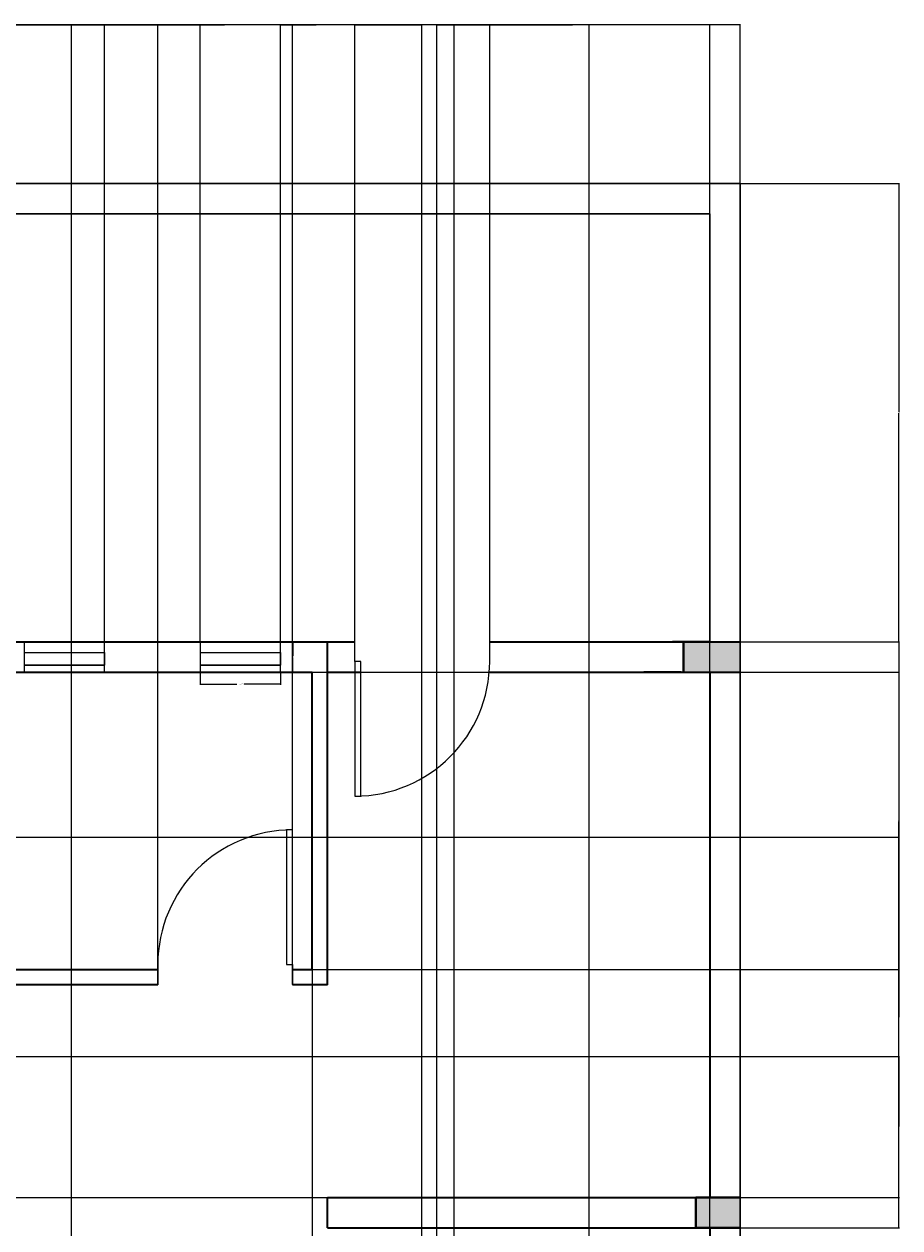
# Model space of a CAD drawing. Units: inches. Extents: x 1210 to 1836, y 84 to 1122.
# Tile 5 of 5: x 1576 to 1836, y 764 to 1122. Entities that reach past the tile are written whole.
import ezdxf

# ---------------------------------------------------------------- set-up
doc = ezdxf.new("R2010")
doc.units = ezdxf.units.IN
doc.header["$MEASUREMENT"] = 0
for name, color, linetype, lineweight in [('A-ANNO-DIMS', 2, 'Continuous', 18), ('A-COLS', 7, 'Continuous', 40), ('A-COLS-PATT', 6, 'Continuous', 13), ('A-GLAZ', 4, 'Continuous', 18), ('A-WALL', 7, 'Continuous', 35), ('C-PROP', 32, 'Continuous', 30), ('DOORS', 24, 'Continuous', 25)]:
    doc.layers.add(name, color=color, linetype=linetype, lineweight=lineweight)
doc.styles.get("Standard").update_dxf_attribs({"font": 'arial.ttf'})
doc.dimstyles.get("Standard").update_dxf_attribs({"dimtxt": 0.18, "dimasz": 0.18, "dimexe": 0.18, "dimexo": 0.0625, "dimgap": 0.09, "dimtad": 0, "dimtih": 1, "dimtoh": 1, "dimdec": 4, "dimzin": 0, "dimdsep": 46, "dimtxsty": 'Standard', "dimcen": 0.09, "dimadec": 0, "dimazin": 0, "dimtfac": 1, "dimtdec": 4, "dimtofl": 0, "dimtmove": 0, "dimatfit": 3, "dimfxl": 1, "dimtolj": 1, "dimtzin": 0, "dimarcsym": 0})

# ---------------------------------------------------------------- blocks, each defined once
blk = doc.blocks.new('*U3')
for p, q in [((0, 0), (0, -6)), ((-40, 0), (-40, -6))]:
    blk.add_line(p, q)
blk.add_lwpolyline([(0, 0), (0, 40), (-1.75, 40), (-1.75, 0)], close=True)
blk.add_arc((0, 0), 40, 90, 180)
blk = doc.blocks.new('*U4')
for p, q in [((0, 0), (0, 6)), ((40, 0), (40, 6))]:
    blk.add_line(p, q)
blk.add_lwpolyline([(0, 0), (0, -40), (1.75, -40), (1.75, 0)], close=True)
blk.add_arc((0, 0), 40, 270, 0)
blk = doc.blocks.new('WIN-24IN')
for p, q in [((0, 9), (0, 0)), ((23.85, 0), (23.85, 9)), ((0.11, 5.82), (23.85, 5.82)), ((23.85, 5.82), (23.85, 2.02)), ((23.85, 2.02), (0, 2.02)), ((0, 2.02), (23.85, 2.02)), ((0, 0), (23.85, 0))]:
    blk.add_line(p, q)
blk = doc.blocks.new('*D20')
at = {"layer": 'A-ANNO-DIMS', "color": 0, "lineweight": -2, "transparency": 16777216}
for p, q in [((1628.07, 929.15), (1628.07, 925.46)), ((1651.92, 929.15), (1651.92, 925.46)), ((1628.25, 925.64), (1638.88, 925.64)), ((1651.74, 925.64), (1641.12, 925.64))]:
    blk.add_line(p, q, dxfattribs=at)
at = {"layer": 'A-ANNO-DIMS', "color": 0, "transparency": 16777216}
for points in [[(1628.25, 925.67), (1628.25, 925.61), (1628.07, 925.64)], [(1651.74, 925.67), (1651.74, 925.61), (1651.92, 925.64)]]:
    blk.add_solid(points, dxfattribs=at)
at = {"layer": 'Defpoints', "color": 0, "transparency": 16777216}
for p in [(1628.07, 929.21), (1651.92, 929.21), (1651.92, 925.64)]:
    blk.add_point(p, dxfattribs=at)
at = {"layer": 'A-ANNO-DIMS', "color": 0, "transparency": 16777216, "insert": (1640, 925.64), "char_height": 0.18, "attachment_point": 5}
blk.add_mtext('\\A1;WINDOW 24 TYP.', dxfattribs=at)
blk = doc.blocks.new('*D21')
at = {"layer": 'A-ANNO-DIMS', "color": 0, "lineweight": -2, "transparency": 16777216}
for p, q in [((1651.99, 938.21), (1655.68, 938.21)), ((1655.5, 938.03), (1655.5, 933.9)), ((1655.5, 929.39), (1655.5, 933.53)), ((1651.99, 929.21), (1655.68, 929.21))]:
    blk.add_line(p, q, dxfattribs=at)
at = {"layer": 'A-ANNO-DIMS', "color": 0, "transparency": 16777216}
for points in [[(1655.47, 938.03), (1655.53, 938.03), (1655.5, 938.21)], [(1655.47, 929.39), (1655.53, 929.39), (1655.5, 929.21)]]:
    blk.add_solid(points, dxfattribs=at)
at = {"layer": 'Defpoints', "color": 0, "transparency": 16777216}
for p in [(1651.92, 938.21), (1655.5, 938.21), (1651.92, 929.21)]:
    blk.add_point(p, dxfattribs=at)
at = {"layer": 'A-ANNO-DIMS', "color": 0, "transparency": 16777216, "insert": (1655.5, 933.71), "char_height": 0.18, "attachment_point": 5}
blk.add_mtext('\\A1;9 TYP.', dxfattribs=at)
blk = doc.blocks.new('*D22')
at = {"layer": 'A-ANNO-DIMS', "color": 0, "lineweight": -2, "transparency": 16777216}
for p, q in [((1257.32, 1074.28), (1257.32, 1121.57)), ((1257.5, 1121.39), (1522.55, 1121.39)), ((1788.14, 1121.39), (1523.1, 1121.39)), ((1788.32, 1074.28), (1788.32, 1121.57))]:
    blk.add_line(p, q, dxfattribs=at)
at = {"layer": 'A-ANNO-DIMS', "color": 0, "transparency": 16777216}
for points in [[(1257.5, 1121.42), (1257.5, 1121.36), (1257.32, 1121.39)], [(1788.14, 1121.42), (1788.14, 1121.36), (1788.32, 1121.39)]]:
    blk.add_solid(points, dxfattribs=at)
at = {"layer": 'Defpoints', "color": 0, "transparency": 16777216}
for p in [(1788.32, 1121.39), (1257.32, 1074.21), (1788.32, 1074.21)]:
    blk.add_point(p, dxfattribs=at)
at = {"layer": 'A-ANNO-DIMS', "color": 0, "transparency": 16777216, "insert": (1522.82, 1121.39), "char_height": 0.18, "attachment_point": 5}
blk.add_mtext('\\A1;531', dxfattribs=at)
blk = doc.blocks.new('*D24')
at = {"layer": 'A-ANNO-DIMS', "color": 0, "lineweight": -2, "transparency": 16777216}
for p, q in [((1788.39, 1074.21), (1835.68, 1074.21)), ((1835.5, 1074.03), (1835.5, 1006.4)), ((1835.5, 938.39), (1835.5, 1006.03)), ((1788.39, 938.21), (1835.68, 938.21))]:
    blk.add_line(p, q, dxfattribs=at)
at = {"layer": 'A-ANNO-DIMS', "color": 0, "transparency": 16777216}
for points in [[(1835.47, 1074.03), (1835.53, 1074.03), (1835.5, 1074.21)], [(1835.47, 938.39), (1835.53, 938.39), (1835.5, 938.21)]]:
    blk.add_solid(points, dxfattribs=at)
at = {"layer": 'Defpoints', "color": 0, "transparency": 16777216}
for p in [(1788.32, 1074.21), (1788.32, 938.21), (1835.5, 938.21)]:
    blk.add_point(p, dxfattribs=at)
at = {"layer": 'A-ANNO-DIMS', "color": 0, "transparency": 16777216, "insert": (1835.5, 1006.21), "char_height": 0.18, "attachment_point": 5}
blk.add_mtext('\\A1;136', dxfattribs=at)
blk = doc.blocks.new('*D25')
at = {"layer": 'A-ANNO-DIMS', "color": 0, "lineweight": -2, "transparency": 16777216}
for p, q in [((1788.39, 938.21), (1835.68, 938.21)), ((1835.5, 938.03), (1835.5, 851.39)), ((1835.5, 764.39), (1835.5, 851.03)), ((1788.39, 764.21), (1835.68, 764.21))]:
    blk.add_line(p, q, dxfattribs=at)
at = {"layer": 'A-ANNO-DIMS', "color": 0, "transparency": 16777216}
for points in [[(1835.47, 938.03), (1835.53, 938.03), (1835.5, 938.21)], [(1835.47, 764.39), (1835.53, 764.39), (1835.5, 764.21)]]:
    blk.add_solid(points, dxfattribs=at)
at = {"layer": 'Defpoints', "color": 0, "transparency": 16777216}
for p in [(1788.32, 938.21), (1788.32, 764.21), (1835.5, 764.21)]:
    blk.add_point(p, dxfattribs=at)
at = {"layer": 'A-ANNO-DIMS', "color": 0, "transparency": 16777216, "insert": (1835.5, 851.21), "char_height": 0.18, "attachment_point": 5}
blk.add_mtext('\\A1;174', dxfattribs=at)
blk = doc.blocks.new('*D36')
at = {"layer": 'A-ANNO-DIMS', "color": 0, "lineweight": -2, "transparency": 16777216}
for p, q in [((1552.32, 840.82), (1552.32, 83.86)), ((1661.32, 840.82), (1661.32, 83.86)), ((1552.5, 84.04), (1606.54, 84.04)), ((1661.14, 84.04), (1607.1, 84.04))]:
    blk.add_line(p, q, dxfattribs=at)
at = {"layer": 'A-ANNO-DIMS', "color": 0, "transparency": 16777216}
for points in [[(1552.5, 84.07), (1552.5, 84.01), (1552.32, 84.04)], [(1661.14, 84.07), (1661.14, 84.01), (1661.32, 84.04)]]:
    blk.add_solid(points, dxfattribs=at)
at = {"layer": 'Defpoints', "color": 0, "transparency": 16777216}
for p in [(1552.32, 840.89), (1661.32, 840.89), (1661.32, 84.04)]:
    blk.add_point(p, dxfattribs=at)
at = {"layer": 'A-ANNO-DIMS', "color": 0, "transparency": 16777216, "insert": (1606.82, 84.04), "char_height": 0.18, "attachment_point": 5}
blk.add_mtext('\\A1;109', dxfattribs=at)
blk = doc.blocks.new('*D37')
at = {"layer": 'A-ANNO-DIMS', "color": 0, "lineweight": -2, "transparency": 16777216}
for p, q in [((1661.39, 929.21), (1835.68, 929.21)), ((1835.5, 929.03), (1835.5, 885.23)), ((1835.5, 841.07), (1835.5, 884.87)), ((1661.39, 840.89), (1835.68, 840.89))]:
    blk.add_line(p, q, dxfattribs=at)
at = {"layer": 'A-ANNO-DIMS', "color": 0, "transparency": 16777216}
for points in [[(1835.47, 929.03), (1835.53, 929.03), (1835.5, 929.21)], [(1835.47, 841.07), (1835.53, 841.07), (1835.5, 840.89)]]:
    blk.add_solid(points, dxfattribs=at)
at = {"layer": 'Defpoints', "color": 0, "transparency": 16777216}
for p in [(1661.32, 929.21), (1661.32, 840.89), (1835.5, 840.89)]:
    blk.add_point(p, dxfattribs=at)
at = {"layer": 'A-ANNO-DIMS', "color": 0, "transparency": 16777216, "insert": (1835.5, 885.05), "char_height": 0.18, "attachment_point": 5}
blk.add_mtext('\\A1;88.33', dxfattribs=at)
blk = doc.blocks.new('*D43')
at = {"layer": 'A-ANNO-DIMS', "color": 0, "lineweight": -2, "transparency": 16777216}
for p, q in [((1375.67, 880.21), (1835.68, 880.21)), ((1835.5, 880.03), (1835.5, 826.9)), ((1835.5, 773.39), (1835.5, 826.53)), ((1375.67, 773.21), (1835.68, 773.21))]:
    blk.add_line(p, q, dxfattribs=at)
at = {"layer": 'A-ANNO-DIMS', "color": 0, "transparency": 16777216}
for points in [[(1835.47, 880.03), (1835.53, 880.03), (1835.5, 880.21)], [(1835.47, 773.39), (1835.53, 773.39), (1835.5, 773.21)]]:
    blk.add_solid(points, dxfattribs=at)
at = {"layer": 'Defpoints', "color": 0, "transparency": 16777216}
for p in [(1375.61, 880.21), (1835.5, 880.21), (1375.61, 773.21)]:
    blk.add_point(p, dxfattribs=at)
at = {"layer": 'A-ANNO-DIMS', "color": 0, "transparency": 16777216, "insert": (1835.5, 826.71), "char_height": 0.18, "attachment_point": 5}
blk.add_mtext('\\A1;107', dxfattribs=at)
blk = doc.blocks.new('*D46')
at = {"layer": 'A-ANNO-DIMS', "color": 0, "lineweight": -2, "transparency": 16777216}
for p, q in [((1543.39, 815.12), (1835.68, 815.12)), ((1835.5, 814.94), (1835.5, 794.35)), ((1835.5, 773.39), (1835.5, 793.98)), ((1543.39, 773.21), (1835.68, 773.21))]:
    blk.add_line(p, q, dxfattribs=at)
at = {"layer": 'A-ANNO-DIMS', "color": 0, "transparency": 16777216}
for points in [[(1835.47, 814.94), (1835.53, 814.94), (1835.5, 815.12)], [(1835.47, 773.39), (1835.53, 773.39), (1835.5, 773.21)]]:
    blk.add_solid(points, dxfattribs=at)
at = {"layer": 'Defpoints', "color": 0, "transparency": 16777216}
for p in [(1543.32, 815.12), (1543.32, 773.21), (1835.5, 773.21)]:
    blk.add_point(p, dxfattribs=at)
at = {"layer": 'A-ANNO-DIMS', "color": 0, "transparency": 16777216, "insert": (1835.5, 794.17), "char_height": 0.18, "attachment_point": 5}
blk.add_mtext('\\A1;41.9', dxfattribs=at)
blk = doc.blocks.new('*D54')
at = {"layer": 'A-ANNO-DIMS', "color": 0, "lineweight": -2, "transparency": 16777216}
for p, q in [((1599.59, 938.28), (1599.59, 1121.57)), ((1599.77, 1121.39), (1613.43, 1121.39)), ((1627.89, 1121.39), (1614.22, 1121.39)), ((1628.07, 938.28), (1628.07, 1121.57))]:
    blk.add_line(p, q, dxfattribs=at)
at = {"layer": 'A-ANNO-DIMS', "color": 0, "transparency": 16777216}
for points in [[(1599.77, 1121.42), (1599.77, 1121.36), (1599.59, 1121.39)], [(1627.89, 1121.42), (1627.89, 1121.36), (1628.07, 1121.39)]]:
    blk.add_solid(points, dxfattribs=at)
at = {"layer": 'Defpoints', "color": 0, "transparency": 16777216}
for p in [(1628.07, 1121.39), (1599.59, 938.21), (1628.07, 938.21)]:
    blk.add_point(p, dxfattribs=at)
at = {"layer": 'A-ANNO-DIMS', "color": 0, "transparency": 16777216, "insert": (1613.83, 1121.39), "char_height": 0.18, "attachment_point": 5}
blk.add_mtext('\\A1;28.48', dxfattribs=at)
blk = doc.blocks.new('*D55')
at = {"layer": 'A-ANNO-DIMS', "color": 0, "lineweight": -2, "transparency": 16777216}
for p, q in [((1651.92, 938.28), (1651.92, 1121.57)), ((1652.1, 1121.39), (1662.49, 1121.39)), ((1673.81, 1121.39), (1663.42, 1121.39)), ((1673.99, 938.28), (1673.99, 1121.57))]:
    blk.add_line(p, q, dxfattribs=at)
at = {"layer": 'A-ANNO-DIMS', "color": 0, "transparency": 16777216}
for points in [[(1652.1, 1121.42), (1652.1, 1121.36), (1651.92, 1121.39)], [(1673.81, 1121.42), (1673.81, 1121.36), (1673.99, 1121.39)]]:
    blk.add_solid(points, dxfattribs=at)
at = {"layer": 'Defpoints', "color": 0, "transparency": 16777216}
for p in [(1673.99, 1121.39), (1651.92, 938.21), (1673.99, 938.21)]:
    blk.add_point(p, dxfattribs=at)
at = {"layer": 'A-ANNO-DIMS', "color": 0, "transparency": 16777216, "insert": (1662.96, 1121.39), "char_height": 0.18, "attachment_point": 5}
blk.add_mtext('\\A1;22.067', dxfattribs=at)
blk = doc.blocks.new('*D56')
at = {"layer": 'A-ANNO-DIMS', "color": 0, "lineweight": -2, "transparency": 16777216}
for p, q in [((1673.99, 938.28), (1673.99, 1121.57)), ((1674.17, 1121.39), (1693.77, 1121.39)), ((1713.81, 1121.39), (1694.21, 1121.39)), ((1713.99, 938.28), (1713.99, 1121.57))]:
    blk.add_line(p, q, dxfattribs=at)
at = {"layer": 'A-ANNO-DIMS', "color": 0, "transparency": 16777216}
for points in [[(1674.17, 1121.42), (1674.17, 1121.36), (1673.99, 1121.39)], [(1713.81, 1121.42), (1713.81, 1121.36), (1713.99, 1121.39)]]:
    blk.add_solid(points, dxfattribs=at)
at = {"layer": 'Defpoints', "color": 0, "transparency": 16777216}
for p in [(1713.99, 1121.39), (1673.99, 938.21), (1713.99, 938.21)]:
    blk.add_point(p, dxfattribs=at)
at = {"layer": 'A-ANNO-DIMS', "color": 0, "transparency": 16777216, "insert": (1693.99, 1121.39), "char_height": 0.18, "attachment_point": 5}
blk.add_mtext('\\A1;40', dxfattribs=at)
blk = doc.blocks.new('*D58')
at = {"layer": 'A-ANNO-DIMS', "color": 0, "lineweight": -2, "transparency": 16777216}
for p, q in [((1615.44, 836.45), (1615.44, 1121.57)), ((1615.62, 1121.39), (1635.22, 1121.39)), ((1655.26, 1121.39), (1635.66, 1121.39)), ((1655.44, 836.45), (1655.44, 1121.57))]:
    blk.add_line(p, q, dxfattribs=at)
at = {"layer": 'A-ANNO-DIMS', "color": 0, "transparency": 16777216}
for points in [[(1615.62, 1121.42), (1615.62, 1121.36), (1615.44, 1121.39)], [(1655.26, 1121.42), (1655.26, 1121.36), (1655.44, 1121.39)]]:
    blk.add_solid(points, dxfattribs=at)
at = {"layer": 'Defpoints', "color": 0, "transparency": 16777216}
for p in [(1655.44, 1121.39), (1615.44, 836.39), (1655.44, 836.39)]:
    blk.add_point(p, dxfattribs=at)
at = {"layer": 'A-ANNO-DIMS', "color": 0, "transparency": 16777216, "insert": (1635.44, 1121.39), "char_height": 0.18, "attachment_point": 5}
blk.add_mtext('\\A1;40', dxfattribs=at)
blk = doc.blocks.new('*D60')
at = {"layer": 'A-ANNO-DIMS', "color": 0, "lineweight": -2, "transparency": 16777216}
for p, q in [((1540.82, 401.28), (1540.82, 1121.57)), ((1541, 1121.39), (1617.04, 1121.39)), ((1693.64, 1121.39), (1617.6, 1121.39)), ((1693.82, 401.28), (1693.82, 1121.57))]:
    blk.add_line(p, q, dxfattribs=at)
at = {"layer": 'A-ANNO-DIMS', "color": 0, "transparency": 16777216}
for points in [[(1541, 1121.42), (1541, 1121.36), (1540.82, 1121.39)], [(1693.64, 1121.42), (1693.64, 1121.36), (1693.82, 1121.39)]]:
    blk.add_solid(points, dxfattribs=at)
at = {"layer": 'Defpoints', "color": 0, "transparency": 16777216}
for p in [(1693.82, 1121.39), (1540.82, 401.21), (1693.82, 401.21)]:
    blk.add_point(p, dxfattribs=at)
at = {"layer": 'A-ANNO-DIMS', "color": 0, "transparency": 16777216, "insert": (1617.32, 1121.39), "char_height": 0.18, "attachment_point": 5}
blk.add_mtext('\\A1;153', dxfattribs=at)
blk = doc.blocks.new('*D61')
at = {"layer": 'A-ANNO-DIMS', "color": 0, "lineweight": -2, "transparency": 16777216}
for p, q in [((1698.32, 412.85), (1698.32, 1121.57)), ((1698.5, 1121.39), (1738.62, 1121.39)), ((1779.14, 1121.39), (1739.03, 1121.39)), ((1779.32, 412.85), (1779.32, 1121.57))]:
    blk.add_line(p, q, dxfattribs=at)
at = {"layer": 'A-ANNO-DIMS', "color": 0, "transparency": 16777216}
for points in [[(1698.5, 1121.42), (1698.5, 1121.36), (1698.32, 1121.39)], [(1779.14, 1121.42), (1779.14, 1121.36), (1779.32, 1121.39)]]:
    blk.add_solid(points, dxfattribs=at)
at = {"layer": 'Defpoints', "color": 0, "transparency": 16777216}
for p in [(1779.32, 1121.39), (1698.32, 412.79), (1779.32, 412.79)]:
    blk.add_point(p, dxfattribs=at)
at = {"layer": 'A-ANNO-DIMS', "color": 0, "transparency": 16777216, "insert": (1738.82, 1121.39), "char_height": 0.18, "attachment_point": 5}
blk.add_mtext('\\A1;81', dxfattribs=at)
blk = doc.blocks.new('*D65')
at = {"layer": 'A-ANNO-DIMS', "color": 0, "lineweight": -2, "transparency": 16777216}
for p, q in [((1549.93, 581.28), (1549.93, 1121.57)), ((1550.11, 1121.39), (1569.48, 1121.39)), ((1589.64, 1121.39), (1570.27, 1121.39)), ((1589.82, 581.28), (1589.82, 1121.57))]:
    blk.add_line(p, q, dxfattribs=at)
at = {"layer": 'A-ANNO-DIMS', "color": 0, "transparency": 16777216}
for points in [[(1550.11, 1121.42), (1550.11, 1121.36), (1549.93, 1121.39)], [(1589.64, 1121.42), (1589.64, 1121.36), (1589.82, 1121.39)]]:
    blk.add_solid(points, dxfattribs=at)
at = {"layer": 'Defpoints', "color": 0, "transparency": 16777216}
for p in [(1589.82, 1121.39), (1549.93, 581.21), (1589.82, 581.21)]:
    blk.add_point(p, dxfattribs=at)
at = {"layer": 'A-ANNO-DIMS', "color": 0, "transparency": 16777216, "insert": (1569.88, 1121.39), "char_height": 0.18, "attachment_point": 5}
blk.add_mtext('\\A1;39.89', dxfattribs=at)
blk = doc.blocks.new('*D77')
at = {"layer": 'A-ANNO-DIMS', "color": 0, "lineweight": -2, "transparency": 16777216}
for p, q in [((1703.49, 496.28), (1703.49, 1121.57)), ((1703.67, 1121.39), (1723.26, 1121.39)), ((1743.31, 1121.39), (1723.71, 1121.39)), ((1743.49, 496.28), (1743.49, 1121.57))]:
    blk.add_line(p, q, dxfattribs=at)
at = {"layer": 'A-ANNO-DIMS', "color": 0, "transparency": 16777216}
for points in [[(1703.67, 1121.42), (1703.67, 1121.36), (1703.49, 1121.39)], [(1743.31, 1121.42), (1743.31, 1121.36), (1743.49, 1121.39)]]:
    blk.add_solid(points, dxfattribs=at)
at = {"layer": 'Defpoints', "color": 0, "transparency": 16777216}
for p in [(1743.49, 1121.39), (1703.49, 496.21), (1743.49, 496.21)]:
    blk.add_point(p, dxfattribs=at)
at = {"layer": 'A-ANNO-DIMS', "color": 0, "transparency": 16777216, "insert": (1723.49, 1121.39), "char_height": 0.18, "attachment_point": 5}
blk.add_mtext('\\A1;40', dxfattribs=at)

msp = doc.modelspace()

# ---------------------------------------------------------------- hatches: boundary and pattern name
at = {"layer": 'A-COLS-PATT'}
h = msp.add_hatch(color=256, dxfattribs=at)
h.dxf.hatch_style = 1
h.paths.add_polyline_path([(1266.3239, 938.214), (1257.3239, 938.214), (1257.3239, 929.4573), (1257.3239, 923.2025), (1266.3239, 923.2025)])
h.paths.add_polyline_path([(1350.3239, 929.214), (1350.3239, 938.214), (1339.1886, 938.214), (1339.1886, 929.214)])
h.paths.add_polyline_path([(1559.1961, 929.214), (1559.1961, 938.214), (1542.8626, 938.214), (1542.8626, 929.214), (1543.3239, 929.214)])
h.paths.add_polyline_path([(1771.5139, 938.214), (1771.5139, 929.214), (1788.3239, 929.214), (1788.3239, 938.214)])
h.paths.add_polyline_path([(1788.3239, 764.214), (1788.3239, 773.214), (1775.2119, 773.214), (1775.2119, 764.214)])
h.paths.add_polyline_path([(1552.3239, 764.214), (1552.3239, 773.214), (1543.3239, 773.214), (1535.8494, 773.197), (1535.8494, 764.214)])
h.paths.add_polyline_path([(1275.5217, 782.2138), (1272.7843, 782.2138), (1266.3239, 782.2138), (1266.3239, 764.214), (1275.5217, 764.214)])
h.paths.add_polyline_path([(1350.2372, 764.214), (1350.3239, 773.214), (1343.6352, 773.214), (1343.6352, 764.214)])
h.paths.add_polyline_path([(1257.3239, 570.3846), (1266.3239, 570.3846), (1266.3239, 590.214), (1257.3239, 590.214)])
h.paths.add_polyline_path([(1450.8239, 572.5809), (1459.8239, 572.5809), (1459.8239, 590.214), (1458.3239, 590.214), (1450.8239, 590.214)])
h.paths.add_polyline_path([(1531.8239, 572.5809), (1540.8239, 572.5809), (1540.8239, 590.214), (1531.8239, 590.214)])
h.paths.add_polyline_path([(1450.8239, 392.214), (1459.8239, 392.214), (1459.8239, 401.214), (1459.8239, 408.7866), (1450.8239, 408.7866)])
h.paths.add_polyline_path([(1531.8239, 392.214), (1540.8239, 392.214), (1540.8239, 401.214), (1540.8239, 408.7866), (1531.8239, 408.7866)])
h.paths.add_polyline_path([(1682.9725, 401.214), (1682.9725, 392.214), (1698.3239, 392.214), (1698.3239, 401.214), (1693.8239, 401.214)])
h.paths.add_polyline_path([(1774.197, 350.714), (1779.3239, 350.714), (1788.3239, 350.714), (1788.3239, 359.714), (1779.3239, 359.714), (1774.197, 359.714)])
h.paths.add_polyline_path([(1779.3239, 590.214), (1775.4485, 590.214), (1775.4485, 581.214), (1779.3239, 581.214), (1788.3239, 581.214), (1788.3239, 590.214)])

# ---------------------------------------------------------------- linework, layer by layer
at = {"layer": 'A-COLS'}
for p, q in [((1771.5139, 938.214), (1771.5139, 929.214)), ((1775.2119, 764.214), (1775.2119, 773.214)), ((1775.2119, 773.214), (1788.3239, 773.214)), ((1775.2119, 764.214), (1788.3239, 764.214))]:
    msp.add_line(p, q, dxfattribs=at)
at = {"layer": 'A-WALL'}
for p, q in [((1266.3239, 938.214), (1673.9914, 938.214)), ((1606.8239, 938.214), (1637.6329, 938.214)), ((1665.8239, 836.3861), (1665.8239, 938.214)), ((1713.9914, 938.214), (1788.3239, 938.214)), ((1779.3239, 938.214), (1768.2524, 938.214)), ((1552.3239, 929.214), (1661.3239, 929.214)), ((1661.3239, 840.8861), (1661.3239, 929.214)), ((1665.8239, 929.214), (1675.7414, 929.214)), ((1713.8651, 929.214), (1788.3239, 929.214)), ((1770.8616, 929.214), (1759.7728, 929.214)), ((1779.3239, 929.214), (1779.3239, 773.214)), ((1552.3239, 840.8861), (1615.4388, 840.8861)), ((1655.4388, 840.8861), (1661.3239, 840.8861)), ((1615.4388, 836.3861), (1552.3239, 836.3861)), ((1665.8239, 836.3861), (1655.4388, 836.3861)), ((1665.8239, 773.214), (1779.3239, 773.214)), ((1665.8239, 764.214), (1665.8239, 773.214)), ((1665.8239, 764.214), (1779.3239, 764.214)), ((1779.3239, 764.214), (1779.3239, 590.214))]:
    msp.add_line(p, q, dxfattribs=at)
at = {"layer": 'C-PROP'}
for p, q in [((1257.3239, 1074.214), (1788.3239, 1074.214)), ((1788.3239, 1074.214), (1788.3239, 131.214)), ((1266.3239, 1065.214), (1779.3239, 1065.214)), ((1779.3239, 1065.214), (1779.3239, 938.214))]:
    msp.add_line(p, q, dxfattribs=at)

# ---------------------------------------------------------------- block references
at = {"layer": 'A-GLAZ'}
for p in [(1575.735, 929.214), (1628.0696, 929.214)]:
    msp.add_blockref('WIN-24IN', p, dxfattribs=at)
at = {"layer": 'DOORS'}
for name, p in [('*U4', (1673.9914, 932.3902)), ('*U3', (1655.4388, 842.3861))]:
    msp.add_blockref(name, p, dxfattribs=at)

# ---------------------------------------------------------------- dimensions: what is measured, and where the dimension line sits
at = {"layer": 'A-ANNO-DIMS'}
for base, p1, p2, override, picture, middle in [((1788.3239, 1121.389), (1257.3239, 1074.214), (1788.3239, 1074.214), {"dimdec": 0, "dimlfac": 1, "dimrnd": 0, "dimzin": 0, "dimdsep": 46, "dimlunit": 2}, '*D22', (1522.8239, 1121.389)), ((1693.8239, 1121.389), (1540.8239, 401.214), (1693.8239, 401.214), {"dimdec": 0, "dimlfac": 1, "dimrnd": 0, "dimzin": 0, "dimdsep": 46, "dimlunit": 2}, '*D60', (1617.3239, 1121.389)), ((1589.8208, 1121.389), (1549.9335, 581.214), (1589.8208, 581.214), {"dimdec": 2, "dimlfac": 1, "dimrnd": 0, "dimzin": 0, "dimdsep": 46, "dimlunit": 2}, '*D65', (1569.8772, 1121.389)), ((1628.0691, 1121.389), (1599.59, 938.214), (1628.0691, 938.214), {"dimdec": 2, "dimlfac": 1, "dimrnd": 0, "dimzin": 0, "dimdsep": 46, "dimlunit": 2}, '*D54', (1613.8295, 1121.389)), ((1655.4388, 1121.389), (1615.4388, 836.3861), (1655.4388, 836.3861), {"dimdec": 0, "dimlfac": 1, "dimrnd": 0, "dimzin": 0, "dimdsep": 46, "dimlunit": 2}, '*D58', (1635.4388, 1121.389)), ((1673.9914, 1121.389), (1651.9245, 938.214), (1673.9914, 938.214), {"dimdec": 3, "dimlfac": 1, "dimrnd": 0, "dimzin": 0, "dimdsep": 46, "dimlunit": 2}, '*D55', (1662.958, 1121.389)), ((1713.9914, 1121.389), (1673.9914, 938.214), (1713.9914, 938.214), {"dimdec": 0, "dimlfac": 1, "dimrnd": 0, "dimzin": 0, "dimdsep": 46, "dimlunit": 2}, '*D56', (1693.9914, 1121.389)), ((1779.3239, 1121.389), (1698.3239, 412.7914), (1779.3239, 412.7914), {"dimdec": 0, "dimlfac": 1, "dimrnd": 0, "dimzin": 0, "dimdsep": 46, "dimlunit": 2}, '*D61', (1738.8239, 1121.389)), ((1743.4865, 1121.389), (1703.4865, 496.214), (1743.4865, 496.214), {"dimdec": 0, "dimlfac": 1, "dimrnd": 0, "dimzin": 0, "dimdsep": 46, "dimlunit": 2}, '*D77', (1723.4865, 1121.389)), ((1661.3239, 84.039), (1552.3239, 840.8861), (1661.3239, 840.8861), {"dimdec": 0, "dimlfac": 1, "dimrnd": 0, "dimzin": 0, "dimdsep": 46, "dimlunit": 2}, '*D36', (1606.8239, 84.039))]:
    dim = msp.add_linear_dim(base=base, p1=p1, p2=p2, dimstyle='Standard', override=override, dxfattribs=at)
    dim.commit()
    dim.dimension.update_dxf_attribs({"geometry": picture, "text_midpoint": middle})
for base, p1, p2, override, picture, middle in [((1835.4989, 938.214), (1788.3239, 1074.214), (1788.3239, 938.214), {"dimdec": 0, "dimlfac": 1, "dimrnd": 0, "dimzin": 0, "dimdsep": 46, "dimlunit": 2}, '*D24', (1835.4989, 1006.214)), ((1835.4989, 764.214), (1788.3239, 938.214), (1788.3239, 764.214), {"dimdec": 0, "dimlfac": 1, "dimrnd": 0, "dimzin": 0, "dimdsep": 46, "dimlunit": 2}, '*D25', (1835.4989, 851.214)), ((1835.4989, 840.8861), (1661.3239, 929.214), (1661.3239, 840.8861), {"dimdec": 2, "dimlfac": 1, "dimrnd": 0, "dimzin": 0, "dimdsep": 46, "dimlunit": 2}, '*D37', (1835.4989, 885.0501)), ((1835.4989, 880.2123), (1375.6096, 773.214), (1375.6096, 880.2123), {"dimdec": 0, "dimlfac": 1, "dimrnd": 0, "dimzin": 0, "dimdsep": 46, "dimlunit": 2}, '*D43', (1835.4989, 826.7132)), ((1835.4989, 773.214), (1543.3239, 815.1167), (1543.3239, 773.214), {"dimdec": 1, "dimlfac": 1, "dimrnd": 0, "dimzin": 0, "dimdsep": 46, "dimlunit": 2}, '*D46', (1835.4989, 794.1654))]:
    dim = msp.add_linear_dim(base=base, p1=p1, p2=p2, angle=90, dimstyle='Standard', override=override, dxfattribs=at)
    dim.commit()
    dim.dimension.update_dxf_attribs({"geometry": picture, "text_midpoint": middle})
dim = msp.add_linear_dim(base=(1655.5028, 938.214), p1=(1651.9245, 929.214), p2=(1651.9245, 938.214), angle=90, text='<> TYP.', dimstyle='Standard', override={"dimdec": 0, "dimlfac": 1, "dimrnd": 0, "dimzin": 0, "dimdsep": 46, "dimlunit": 2}, dxfattribs=at)
dim.commit()
dim.dimension.update_dxf_attribs({"geometry": '*D21', "text_midpoint": (1655.5028, 933.714)})
dim = msp.add_linear_dim(base=(1651.9245, 925.6357), p1=(1628.0691, 929.214), p2=(1651.9245, 929.214), text='WINDOW <> TYP.', dimstyle='Standard', override={"dimdec": 0, "dimlfac": 1, "dimrnd": 0, "dimzin": 0, "dimdsep": 46, "dimlunit": 2}, dxfattribs=at)
dim.commit()
dim.dimension.update_dxf_attribs({"geometry": '*D20', "text_midpoint": (1639.9968, 925.6357)})

doc.saveas('drawing.dxf')
